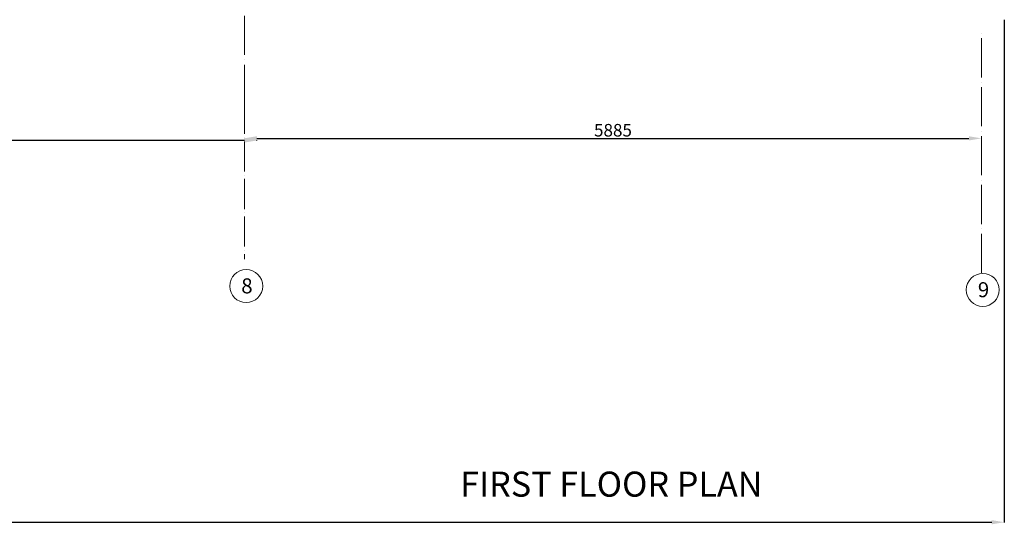
# Model space of a CAD drawing. Units: millimetres. Extents: x -3326 to 29338, y -16792 to 6002.
# Tile 14 of 21: x 21421 to 29282, y -16792 to -12764. Entities that reach past the tile are written whole.
import ezdxf

# ---------------------------------------------------------------- set-up
doc = ezdxf.new("R2010")
doc.units = ezdxf.units.MM
doc.header["$PDMODE"] = 35
doc.header["$PDSIZE"] = 5
doc.linetypes.add('ACAD_ISO04W100', pattern=[30, 24, -3, 0, -3])
for name, color, linetype, lineweight in [('A-ANNO-DIMS', 2, 'Continuous', 13), ('A-ANNO-TTLB', 7, 'Continuous', 35), ('A-GRID', 8, 'ACAD_ISO04W100', 13), ('A-GRID-IDEN', 7, 'Continuous', 18)]:
    doc.layers.add(name, color=color, linetype=linetype, lineweight=lineweight)
doc.styles.get("Standard").update_dxf_attribs({"font": 'arial.ttf'})
doc.dimstyles.new('ISO-25', dxfattribs={"dimtxt": 100, "dimasz": 100, "dimexe": 1.25, "dimexo": 0.625, "dimtad": 1, "dimtxsty": 'Standard', "dimcen": 2.5, "dimadec": 0, "dimazin": 0, "dimtfac": 1, "dimtmove": 0, "dimatfit": 3, "dimfxl": 1, "dimarcsym": 0})

# ---------------------------------------------------------------- blocks, each defined once
blk = doc.blocks.new('*D157')
at = {"layer": 'A-ANNO-DIMS', "color": 0, "lineweight": -2, "transparency": 16777216}
for p, q in [((23215, -13710.3), (23215, -13709.6)), ((23315, -13710.9), (29000, -13710.9)), ((29100, -13710.3), (29100, -13709.6))]:
    blk.add_line(p, q, dxfattribs=at)
at = {"layer": 'A-ANNO-DIMS', "color": 0, "transparency": 16777216}
for points in [[(23315, -13694.2), (23315, -13727.6), (23215, -13710.9)], [(29000, -13694.2), (29000, -13727.6), (29100, -13710.9)]]:
    blk.add_solid(points, dxfattribs=at)
at = {"layer": 'Defpoints', "color": 0, "transparency": 16777216}
for p in [(23215, -13710.9), (29100, -13710.9), (29100, -13710.9)]:
    blk.add_point(p, dxfattribs=at)
at = {"layer": 'A-ANNO-DIMS', "color": 0, "transparency": 16777216, "insert": (26157.5, -13659.2), "char_height": 100, "attachment_point": 5}
blk.add_mtext('5885', dxfattribs=at)
blk = doc.blocks.new('*D158')
at = {"layer": 'A-ANNO-DIMS', "color": 0, "lineweight": -2, "transparency": 16777216}
for p, q in [((17245, -13726.9), (17245, -13726.3)), ((23215, -13727.6), (17345, -13727.6)), ((23315, -13726.9), (23315, -13726.3))]:
    blk.add_line(p, q, dxfattribs=at)
at = {"layer": 'A-ANNO-DIMS', "color": 0, "transparency": 16777216}
for points in [[(17345, -13710.9), (17345, -13744.2), (17245, -13727.6)], [(23215, -13710.9), (23215, -13744.2), (23315, -13727.6)]]:
    blk.add_solid(points, dxfattribs=at)
at = {"layer": 'Defpoints', "color": 0, "transparency": 16777216}
for p in [(17245, -13727.6), (17245, -13727.6), (23315, -13727.6)]:
    blk.add_point(p, dxfattribs=at)
at = {"layer": 'A-ANNO-DIMS', "color": 0, "transparency": 16777216, "insert": (20280, -13675.9), "char_height": 100, "attachment_point": 5}
blk.add_mtext('6070', dxfattribs=at)
blk = doc.blocks.new('*D235')
at = {"layer": 'A-ANNO-DIMS', "color": 0, "lineweight": -2, "transparency": 16777216}
for p, q in [((-617.7, -12764.6), (-617.7, -16776.1)), ((29282.3, -12764.6), (29282.3, -16776.1)), ((-517.7, -16774.9), (29182.3, -16774.9))]:
    blk.add_line(p, q, dxfattribs=at)
at = {"layer": 'A-ANNO-DIMS', "color": 0, "transparency": 16777216}
for points in [[(-517.7, -16758.2), (-517.7, -16791.6), (-617.7, -16774.9)], [(29182.3, -16758.2), (29182.3, -16791.6), (29282.3, -16774.9)]]:
    blk.add_solid(points, dxfattribs=at)
at = {"layer": 'Defpoints', "color": 0, "transparency": 16777216}
for p in [(-617.7, -12764), (29282.3, -12764), (29282.3, -16774.9)]:
    blk.add_point(p, dxfattribs=at)
at = {"layer": 'A-ANNO-DIMS', "color": 0, "transparency": 16777216, "insert": (14332.3, -16723.2), "char_height": 100, "attachment_point": 5}
blk.add_mtext('29900', dxfattribs=at)

msp = doc.modelspace()

# ---------------------------------------------------------------- linework, layer by layer
at = {"layer": 'A-GRID', "ltscale": 13}
for p, q in [((23214.966, -13434.889), (23214.966, -11505.956)), ((29099.966, -14784.889), (29099.966, -12855.956))]:
    msp.add_line(p, q, dxfattribs=at)
at = {"layer": 'A-GRID', "ltscale": 10}
msp.add_line((23214.966, -13434.889), (23214.966, -14674.996), dxfattribs=at)
at = {"layer": 'A-GRID-IDEN'}
for centre, radius in [((23229.016, -14889.669), 131.577), ((29110.456, -14920.492), 131.527)]:
    msp.add_circle(centre, radius, dxfattribs=at)

# ---------------------------------------------------------------- texts
at = {"layer": 'A-ANNO-TTLB', "insert": (24937.969, -16370.89), "char_height": 200, "attachment_point": 1}
msp.add_mtext_dynamic_manual_height_columns('FIRST FLOOR PLAN', width=10814.3674, gutter_width=12.5, heights=[0], dxfattribs=at)
at = {"layer": 'A-GRID-IDEN', "char_height": 120, "attachment_point": 1}
for s, heights, insert in [('8', [0], (23189.48, -14828.4)), ('9', [204.477], (29071.002, -14859.223))]:
    msp.add_mtext_dynamic_manual_height_columns(s, width=463.74815, gutter_width=12.5, heights=heights, dxfattribs=dict(at, insert=insert))

# ---------------------------------------------------------------- dimensions: what is measured, and where the dimension line sits
at = {"layer": 'A-ANNO-DIMS'}
for base, p1, p2, override, picture, middle in [((29282.301, -16774.892), (-617.699, -12763.952), (29282.301, -12763.952), {"dimdec": 0, "dimlfac": 1, "dimrnd": 0, "dimzin": 0, "dimdsep": 46, "dimlunit": 2}, '*D235', (14332.301, -16723.21)), ((29099.966, -13710.895), (23214.966, -13710.895), (29099.966, -13710.895), {"dimclrd": 0, "dimclre": 0, "dimclrt": 0}, '*D157', (26157.466, -13659.213)), ((17244.966, -13727.562), (23314.966, -13727.562), (17244.966, -13727.562), {"dimclrd": 0, "dimclre": 0, "dimclrt": 0}, '*D158', (20279.966, -13675.88))]:
    dim = msp.add_linear_dim(base=base, p1=p1, p2=p2, dimstyle='ISO-25', override=override, dxfattribs=at)
    dim.commit()
    dim.dimension.update_dxf_attribs({"geometry": picture, "text_midpoint": middle})

doc.saveas('drawing.dxf')
